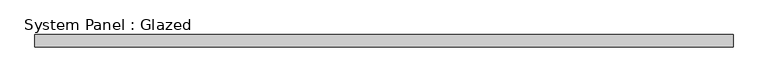
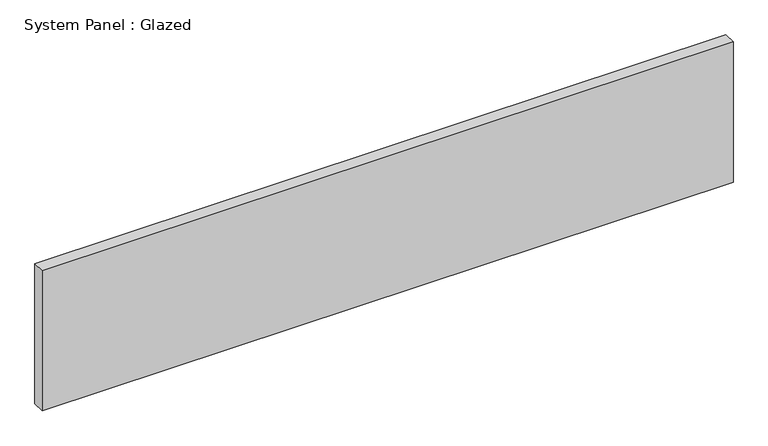
"""IFC4 building model written with IfcOpenShell, lengths in millimetres: plate geometry, System Panel : Glazed."""

from ifc_helpers import new_model, si_unit, origin, origin_with_axes, place, context, project, spatial, polyline, outline, extrude, source, transform, mapped, element, save


def system_panel_glazed_d663d970(model_context):
    return source(origin(), model_context, "Body", "SweptSolid", [
        extrude(outline(polyline([(711.2, 19.05), (-711.2, 19.05), (-711.2, 44.45), (711.2, 44.45), (711.2, 19.05)])), origin_with_axes(), (0.0, 0.0, 1.0), 304.8),
    ])


if __name__ == "__main__":
    model = new_model("IFC4")
    model_context = context("Model", 3, world=origin())
    ifc_project = project(units=[si_unit("LENGTHUNIT", "METRE", prefix="MILLI")], contexts=[model_context])
    site = spatial("IfcSite", under=ifc_project)
    building = spatial("IfcBuilding", under=site)
    placement = place(None, origin())
    system_panel_glazed_shape = system_panel_glazed_d663d970(model_context)
    element("IfcPlate", 1, ObjectType="System Panel : Glazed", at=placement, inside=building, context=model_context, shape_type="MappedRepresentation", body=[
        mapped(system_panel_glazed_shape, transform((0.0, 0.0, 0.0), x_axis=(1.0, 0.0, 0.0), y_axis=(0.0, 1.0, 0.0), z_axis=(0.0, 0.0, 1.0))),
    ])
    save(model, "model.ifc")

# Revit data of these elements
# Type "System Panel : Glazed"
#   Construction Type Id = "GSP4R"
#   Analytic Construction = "1/8 in Pilkington single glazing"
#   Visual Light Transmittance = 0.9
#   Solar Heat Gain Coefficient = 0.86
#   Heat Transfer Coefficient (U) = 1.18115 BTU/(h·ft²·°F)
#   Define Thermal Properties by = 1
# Element 1 (IfcPlate, "System Panel : Glazed")
#   Materials on its faces: "Glass"
# Materials
#   "Glass": class "Glass", colour RGB 0 128 192, transparency 0.75, Description = "Soda Lime Glass", Cost = 0
